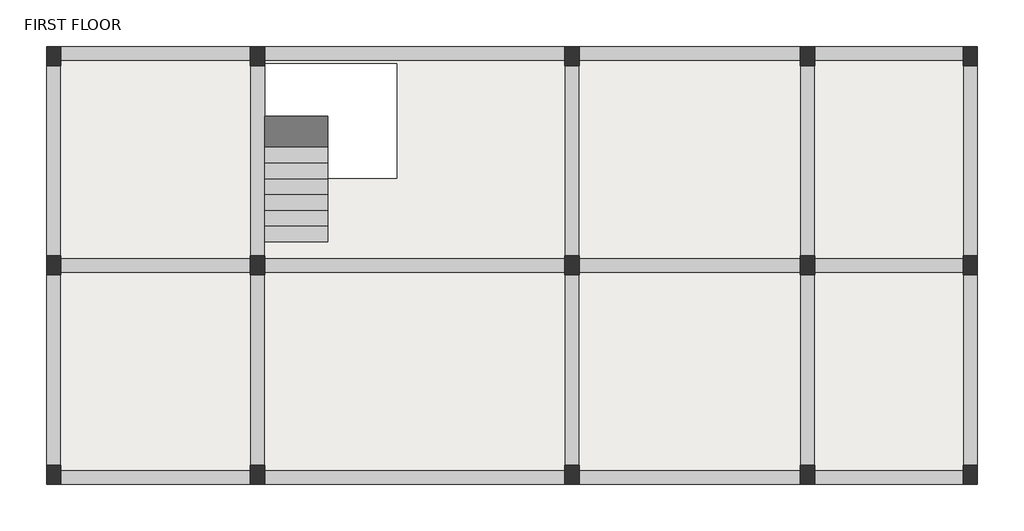
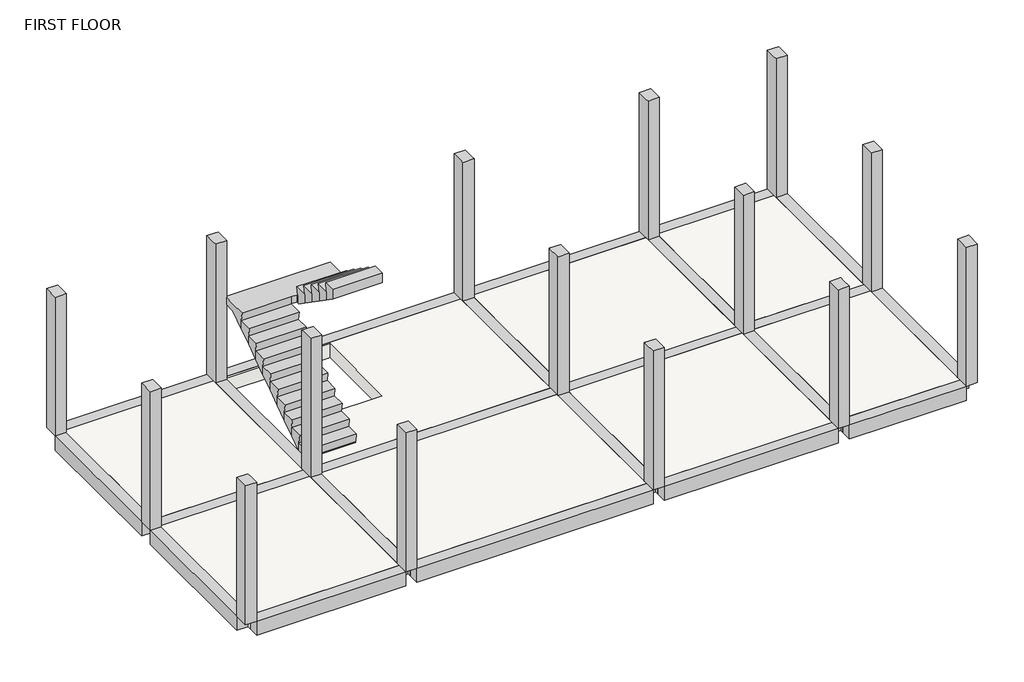
# One storey: 22 beams, 15 columns, 2 slabs, 1 stair flight.
"""IFC4 building model written with IfcOpenShell, lengths in millimetres."""

from ifc_helpers import new_model, si_unit, frame, origin, place, context, project, spatial, polyline, outline, extrude, faceted_brep, element, save

model = new_model("IFC4")

# Units and contexts
model_context = context("Model", 3, world=origin())
ifc_project = project(units=[si_unit("LENGTHUNIT", "METRE", prefix="MILLI")], contexts=[model_context])

# Site, building, storey
site = spatial("IfcSite", under=ifc_project)
building = spatial("IfcBuilding", under=site)
storey = spatial("IfcBuildingStorey", under=building, Name="FIRST FLOOR", Elevation=3000.0)

# Beams
placement = place(None, origin())
element("IfcBeam", 1, ObjectType="M_Concrete-Rectangular Beam : 100MM X 200MM", at=placement, inside=storey, context=model_context, shape_type="SweptSolid", body=[
    extrude(outline(polyline([(-5114.1068817, 5712.0180792), (-5342.7068817, 5712.0180792), (-5342.7068817, 8772.8765586), (-5114.1068817, 8772.8765586), (-5114.1068817, 5712.0180792)])), frame((0.0, 0.0, 2695.2), z_axis=(0.0, 0.0, 1.0), x_axis=(1.0, 0.0, 0.0)), (0.0, 0.0, 1.0), 304.8),
])
element("IfcBeam", 2, ObjectType="M_Concrete-Rectangular Beam : 100MM X 200MM", at=placement, inside=storey, context=model_context, shape_type="Brep", body=[
    faceted_brep([(-2066.1068817, 2041.8765586, 3000.0), (-2066.1068817, 2270.4765586, 3000.0), (-5114.1068817, 2270.4765586, 3000.0), (-5114.1068817, 2041.8765586, 3000.0), (-2066.1068817, 2041.8765586, 2695.2), (-5114.1068817, 2041.8765586, 2695.2), (-2066.1068817, 2270.4765586, 2695.2), (-5114.1068817, 2270.4765586, 2695.2), (-2066.1068817, 2270.4765586, 2700.0), (-5114.1068817, 2270.4765586, 2700.0)], [[[0, 1, 2, 3]], [[4, 0, 3, 5]], [[6, 4, 5, 7]], [[1, 8, 6, 7, 9, 2]], [[1, 0, 4, 6, 8]], [[3, 2, 9, 7, 5]]]),
])
element("IfcBeam", 3, ObjectType="M_Concrete-Rectangular Beam : 100MM X 200MM", at=placement, inside=storey, context=model_context, shape_type="SweptSolid", body=[
    extrude(outline(polyline([(-5114.1068817, 2346.6765586), (-5342.7068817, 2346.6765586), (-5342.7068817, 5407.2180792), (-5114.1068817, 5407.2180792), (-5114.1068817, 2346.6765586)])), frame((0.0, 0.0, 2695.2), z_axis=(0.0, 0.0, 1.0), x_axis=(1.0, 0.0, 0.0)), (0.0, 0.0, 1.0), 304.8),
])
element("IfcBeam", 4, ObjectType="M_Concrete-Rectangular Beam : 100MM X 200MM", at=placement, inside=storey, context=model_context, shape_type="Brep", body=[
    faceted_brep([(2988.1931183, 2041.8765586, 3000.0), (2988.1931183, 2270.4765586, 3000.0), (-1837.5068817, 2270.4765586, 3000.0), (-1837.5068817, 2041.8765586, 3000.0), (2988.1931183, 2041.8765586, 2695.2), (-1837.5068817, 2041.8765586, 2695.2), (2988.1931183, 2270.4765586, 2695.2), (-1837.5068817, 2270.4765586, 2695.2), (-1837.5068817, 2270.4765586, 2700.0)], [[[0, 1, 2, 3]], [[4, 0, 3, 5]], [[6, 4, 5, 7]], [[1, 6, 7, 8, 2]], [[1, 0, 4, 6]], [[3, 2, 8, 7, 5]]]),
])
element("IfcBeam", 5, ObjectType="M_Concrete-Rectangular Beam : 100MM X 200MM", at=placement, inside=storey, context=model_context, shape_type="Brep", body=[
    faceted_brep([(6773.0931183, 2041.8765586, 3000.0), (6773.0931183, 2270.4765586, 3000.0), (3217.0931183, 2270.4765586, 3000.0), (3217.0931183, 2041.8765586, 3000.0), (6773.0931183, 2041.8765586, 2695.2), (3217.0931183, 2041.8765586, 2695.2), (6773.0931183, 2270.4765586, 2695.2), (3217.0931183, 2270.4765586, 2695.2), (6773.0931183, 2270.4765586, 2700.0), (3217.0931183, 2270.4765586, 2700.0)], [[[0, 1, 2, 3]], [[4, 0, 3, 5]], [[6, 4, 5, 7]], [[1, 8, 6, 7, 9, 2]], [[1, 0, 4, 6, 8]], [[3, 2, 9, 7, 5]]]),
])
element("IfcBeam", 6, ObjectType="M_Concrete-Rectangular Beam : 100MM X 200MM", at=placement, inside=storey, context=model_context, shape_type="Brep", body=[
    faceted_brep([(9387.3931183, 2041.8765586, 3000.0), (9387.3931183, 2270.4765586, 3000.0), (7001.6931183, 2270.4765586, 3000.0), (7001.6931183, 2041.8765586, 3000.0), (9387.3931183, 2041.8765586, 2695.2), (7001.6931183, 2041.8765586, 2695.2), (9387.3931183, 2270.4765586, 2695.2), (7001.6931183, 2270.4765586, 2695.2), (7001.6931183, 2270.4765586, 2700.0)], [[[0, 1, 2, 3]], [[4, 0, 3, 5]], [[6, 4, 5, 7]], [[1, 6, 7, 8, 2]], [[1, 0, 4, 6]], [[3, 2, 8, 7, 5]]]),
])
element("IfcBeam", 7, ObjectType="M_Concrete-Rectangular Beam : 100MM X 200MM", at=placement, inside=storey, context=model_context, shape_type="Brep", body=[
    faceted_brep([(-2066.1068817, 8849.0765586, 3000.0), (-2066.1068817, 9077.6765586, 3000.0), (-5114.1068817, 9077.6765586, 3000.0), (-5114.1068817, 8849.0765586, 3000.0), (-2066.1068817, 8849.0765586, 2695.2), (-2066.1068817, 8849.0765586, 2700.0), (-5114.1068817, 8849.0765586, 2700.0), (-5114.1068817, 8849.0765586, 2695.2), (-2066.1068817, 9077.6765586, 2695.2), (-5114.1068817, 9077.6765586, 2695.2)], [[[0, 1, 2, 3]], [[4, 5, 0, 3, 6, 7]], [[8, 4, 7, 9]], [[1, 8, 9, 2]], [[1, 0, 5, 4, 8]], [[3, 2, 9, 7, 6]]]),
])
element("IfcBeam", 8, ObjectType="M_Concrete-Rectangular Beam : 100MM X 200MM", at=placement, inside=storey, context=model_context, shape_type="Brep", body=[
    faceted_brep([(2988.4931183, 8849.0765586, 3000.0), (2988.4931183, 9077.6765586, 3000.0), (-1837.5068817, 9077.6765586, 3000.0), (-1837.5068817, 8849.0765586, 3000.0), (2988.4931183, 8849.0765586, 2695.2), (2988.4931183, 8849.0765586, 2700.0), (-1837.5068817, 8849.0765586, 2700.0), (-1837.5068817, 8849.0765586, 2695.2), (2988.4931183, 9077.6765586, 2695.2), (-1837.5068817, 9077.6765586, 2695.2)], [[[0, 1, 2, 3]], [[4, 5, 0, 3, 6, 7]], [[8, 4, 7, 9]], [[1, 8, 9, 2]], [[1, 0, 5, 4, 8]], [[3, 2, 9, 7, 6]]]),
])
element("IfcBeam", 9, ObjectType="M_Concrete-Rectangular Beam : 100MM X 200MM", at=placement, inside=storey, context=model_context, shape_type="Brep", body=[
    faceted_brep([(6773.0931183, 8849.0765586, 3000.0), (6773.0931183, 9077.6765586, 3000.0), (3217.0931183, 9077.6765586, 3000.0), (3217.0931183, 8849.0765586, 3000.0), (6773.0931183, 8849.0765586, 2695.2), (6773.0931183, 8849.0765586, 2700.0), (3217.0931183, 8849.0765586, 2700.0), (3217.0931183, 8849.0765586, 2695.2), (6773.0931183, 9077.6765586, 2695.2), (3217.0931183, 9077.6765586, 2695.2)], [[[0, 1, 2, 3]], [[4, 5, 0, 3, 6, 7]], [[8, 4, 7, 9]], [[1, 8, 9, 2]], [[1, 0, 5, 4, 8]], [[3, 2, 9, 7, 6]]]),
])
element("IfcBeam", 10, ObjectType="M_Concrete-Rectangular Beam : 100MM X 200MM", at=placement, inside=storey, context=model_context, shape_type="Brep", body=[
    faceted_brep([(9387.3931183, 8849.0765586, 3000.0), (9387.3931183, 9077.6765586, 3000.0), (7001.6931183, 9077.6765586, 3000.0), (7001.6931183, 8849.0765586, 3000.0), (9387.3931183, 8849.0765586, 2695.2), (7001.6931183, 8849.0765586, 2700.0), (7001.6931183, 8849.0765586, 2695.2), (9387.3931183, 9077.6765586, 2695.2), (7001.6931183, 9077.6765586, 2695.2)], [[[0, 1, 2, 3]], [[4, 0, 3, 5, 6]], [[7, 4, 6, 8]], [[1, 7, 8, 2]], [[1, 0, 4, 7]], [[3, 2, 8, 6, 5]]]),
])
element("IfcBeam", 11, ObjectType="M_Concrete-Rectangular Beam : 100MM X 200MM", at=placement, inside=storey, context=model_context, shape_type="SweptSolid", body=[
    extrude(outline(polyline([(9617.8931183, 2354.2765586), (9389.2931183, 2354.2765586), (9389.2931183, 5407.2180792), (9617.8931183, 5407.2180792), (9617.8931183, 2354.2765586)])), frame((0.0, 0.0, 2695.2), z_axis=(0.0, 0.0, 1.0), x_axis=(1.0, 0.0, 0.0)), (0.0, 0.0, 1.0), 304.8),
])
element("IfcBeam", 12, ObjectType="M_Concrete-Rectangular Beam : 100MM X 200MM", at=placement, inside=storey, context=model_context, shape_type="SweptSolid", body=[
    extrude(outline(polyline([(9389.2931183, 8772.8765586), (9617.8931183, 8772.8765586), (9617.8931183, 5712.0180792), (9389.2931183, 5712.0180792), (9389.2931183, 8772.8765586)])), frame((0.0, 0.0, 2695.2), z_axis=(0.0, 0.0, 1.0), x_axis=(1.0, 0.0, 0.0)), (0.0, 0.0, 1.0), 304.8),
])
element("IfcBeam", 13, ObjectType="M_Concrete-Rectangular Beam : 100MM X 200MM", at=placement, inside=storey, context=model_context, shape_type="Brep", body=[
    faceted_brep([(7001.6931183, 5445.3180792, 3000.0), (9389.2931183, 5445.3180792, 3000.0), (9389.2931183, 5673.9180792, 3000.0), (7001.6931183, 5673.9180792, 3000.0), (9389.2931183, 5673.9180792, 2700.0), (9389.2931183, 5673.9180792, 2695.2), (7001.6931183, 5673.9180792, 2695.2), (7001.6931183, 5673.9180792, 2700.0), (9389.2931183, 5445.3180792, 2695.2), (7001.6931183, 5445.3180792, 2695.2), (7001.6931183, 5445.3180792, 2700.0), (9389.2931183, 5445.3180792, 2700.0)], [[[0, 1, 2, 3]], [[3, 2, 4, 5, 6, 7]], [[5, 8, 9, 6]], [[1, 0, 10, 9, 8, 11]], [[5, 4, 2, 1, 11, 8]], [[0, 3, 7, 6, 9, 10]]]),
])
element("IfcBeam", 14, ObjectType="M_Concrete-Rectangular Beam : 100MM X 200MM", at=placement, inside=storey, context=model_context, shape_type="Brep", body=[
    faceted_brep([(3217.0931183, 5445.3180792, 3000.0), (6773.0931183, 5445.3180792, 3000.0), (6773.0931183, 5673.9180792, 3000.0), (3217.0931183, 5673.9180792, 3000.0), (6773.0931183, 5673.9180792, 2700.0), (6773.0931183, 5673.9180792, 2695.2), (3217.0931183, 5673.9180792, 2695.2), (3217.0931183, 5673.9180792, 2700.0), (6773.0931183, 5445.3180792, 2695.2), (3217.0931183, 5445.3180792, 2695.2), (3217.0931183, 5445.3180792, 2700.0), (6773.0931183, 5445.3180792, 2700.0)], [[[0, 1, 2, 3]], [[3, 2, 4, 5, 6, 7]], [[5, 8, 9, 6]], [[1, 0, 10, 9, 8, 11]], [[2, 1, 11, 8, 5, 4]], [[0, 3, 7, 6, 9, 10]]]),
])
element("IfcBeam", 15, ObjectType="M_Concrete-Rectangular Beam : 100MM X 200MM", at=placement, inside=storey, context=model_context, shape_type="Brep", body=[
    faceted_brep([(-1837.5068817, 5445.3180792, 3000.0), (2988.4931183, 5445.3180792, 3000.0), (2988.4931183, 5673.9180792, 3000.0), (-1837.5068817, 5673.9180792, 3000.0), (2988.4931183, 5673.9180792, 2700.0), (2988.4931183, 5673.9180792, 2695.2), (-1837.5068817, 5673.9180792, 2695.2), (-1837.5068817, 5673.9180792, 2700.0), (2988.4931183, 5445.3180792, 2695.2), (-1837.5068817, 5445.3180792, 2695.2), (-1837.5068817, 5445.3180792, 2700.0), (2988.4931183, 5445.3180792, 2700.0)], [[[0, 1, 2, 3]], [[3, 2, 4, 5, 6, 7]], [[5, 8, 9, 6]], [[1, 0, 10, 9, 8, 11]], [[2, 1, 11, 8, 5, 4]], [[0, 3, 7, 6, 9, 10]]]),
])
element("IfcBeam", 16, ObjectType="M_Concrete-Rectangular Beam : 100MM X 200MM", at=placement, inside=storey, context=model_context, shape_type="Brep", body=[
    faceted_brep([(-2066.1068817, 5673.9180792, 3000.0), (-5114.1068817, 5673.9180792, 3000.0), (-5114.1068817, 5445.3180792, 3000.0), (-2066.1068817, 5445.3180792, 3000.0), (-2066.1068817, 5673.9180792, 2700.0), (-2066.1068817, 5673.9180792, 2695.2), (-5114.1068817, 5673.9180792, 2695.2), (-5114.1068817, 5673.9180792, 2700.0), (-2066.1068817, 5445.3180792, 2695.2), (-5114.1068817, 5445.3180792, 2695.2), (-2066.1068817, 5445.3180792, 2700.0), (-5114.1068817, 5445.3180792, 2700.0)], [[[0, 1, 2, 3]], [[1, 0, 4, 5, 6, 7]], [[5, 8, 9, 6]], [[8, 10, 3, 2, 11, 9]], [[0, 3, 10, 8, 5, 4]], [[2, 1, 7, 6, 9, 11]]]),
])
element("IfcBeam", 17, ObjectType="M_Concrete-Rectangular Beam : 100MM X 200MM", at=placement, inside=storey, context=model_context, shape_type="SweptSolid", body=[
    extrude(outline(polyline([(6773.0931183, 5407.2180792), (7001.6931183, 5407.2180792), (7001.6931183, 2346.6765586), (6773.0931183, 2346.6765586), (6773.0931183, 5407.2180792)])), frame((0.0, 0.0, 2695.2), z_axis=(0.0, 0.0, 1.0), x_axis=(1.0, 0.0, 0.0)), (0.0, 0.0, 1.0), 304.8),
])
element("IfcBeam", 18, ObjectType="M_Concrete-Rectangular Beam : 100MM X 200MM", at=placement, inside=storey, context=model_context, shape_type="SweptSolid", body=[
    extrude(outline(polyline([(6773.0931183, 8772.8765586), (7001.6931183, 8772.8765586), (7001.6931183, 5712.0180792), (6773.0931183, 5712.0180792), (6773.0931183, 8772.8765586)])), frame((0.0, 0.0, 2695.2), z_axis=(0.0, 0.0, 1.0), x_axis=(1.0, 0.0, 0.0)), (0.0, 0.0, 1.0), 304.8),
])
element("IfcBeam", 19, ObjectType="M_Concrete-Rectangular Beam : 100MM X 200MM", at=placement, inside=storey, context=model_context, shape_type="SweptSolid", body=[
    extrude(outline(polyline([(2988.4931183, 5407.2180792), (3217.0931183, 5407.2180792), (3217.0931183, 2346.6765586), (2988.4931183, 2346.6765586), (2988.4931183, 5407.2180792)])), frame((0.0, 0.0, 2695.2), z_axis=(0.0, 0.0, 1.0), x_axis=(1.0, 0.0, 0.0)), (0.0, 0.0, 1.0), 304.8),
])
element("IfcBeam", 20, ObjectType="M_Concrete-Rectangular Beam : 100MM X 200MM", at=placement, inside=storey, context=model_context, shape_type="Brep", body=[
    faceted_brep([(2988.4931183, 5719.6180792, 3000.0), (3217.0931183, 5719.6180792, 3000.0), (3217.0931183, 8772.8765586, 3000.0), (2988.4931183, 8772.8765586, 3000.0), (3217.0931183, 5719.6180792, 2700.0), (3217.0931183, 5719.6180792, 2695.2), (3217.0931183, 8772.8765586, 2695.2), (2988.4931183, 5719.6180792, 2695.2), (2988.4931183, 8772.8765586, 2695.2), (2988.4931183, 5719.6180792, 2700.0)], [[[0, 1, 2, 3]], [[1, 4, 5, 6, 2]], [[5, 7, 8, 6]], [[7, 9, 0, 3, 8]], [[7, 5, 4, 1, 0, 9]], [[3, 2, 6, 8]]]),
])
element("IfcBeam", 21, ObjectType="M_Concrete-Rectangular Beam : 100MM X 200MM", at=placement, inside=storey, context=model_context, shape_type="SweptSolid", body=[
    extrude(outline(polyline([(-2066.1068817, 5407.2180792), (-1837.5068817, 5407.2180792), (-1837.5068817, 2346.6765586), (-2066.1068817, 2346.6765586), (-2066.1068817, 5407.2180792)])), frame((0.0, 0.0, 2695.2), z_axis=(0.0, 0.0, 1.0), x_axis=(1.0, 0.0, 0.0)), (0.0, 0.0, 1.0), 304.8),
])
element("IfcBeam", 22, ObjectType="M_Concrete-Rectangular Beam : 100MM X 200MM", at=placement, inside=storey, context=model_context, shape_type="Brep", body=[
    faceted_brep([(-1837.5068817, 8772.8765586, 3000.0), (-2066.1068817, 8772.8765586, 3000.0), (-2066.1068817, 5712.0180792, 3000.0), (-1837.5068817, 5712.0180792, 3000.0), (-1837.5068817, 5940.7765586, 3000.0), (-1837.5068817, 8772.8765586, 2695.2), (-1837.5068817, 5712.0180792, 2695.2), (-2066.1068817, 8772.8765586, 2695.2), (-2066.1068817, 5712.0180792, 2695.2)], [[[0, 1, 2, 3, 4]], [[5, 0, 4, 3, 6]], [[7, 5, 6, 8]], [[1, 7, 8, 2]], [[1, 0, 5, 7]], [[3, 2, 8, 6]]]),
])

# Columns
element("IfcColumn", 23, ObjectType="M_Concrete-Rectangular-Column : 9\" X 1' COLUMNS", at=placement, inside=storey, context=model_context, shape_type="Brep", body=[
    faceted_brep([(9617.8931183, 9077.6765586, 3000.0), (9617.8931183, 8772.8765586, 3000.0), (9389.2931183, 8772.8765586, 3000.0), (9389.2931183, 9077.6765586, 3000.0), (9617.8931183, 9077.6765586, 6000.0), (9617.8931183, 8772.8765586, 6000.0), (9389.2931183, 8772.8765586, 6000.0), (9389.2931183, 8849.0765586, 6000.0), (9389.2931183, 9077.6765586, 6000.0)], [[[0, 1, 2, 3]], [[4, 5, 1, 0]], [[5, 6, 2, 1]], [[6, 7, 8, 3, 2]], [[8, 4, 0, 3]], [[4, 8, 7, 6, 5]]]),
])
element("IfcColumn", 24, ObjectType="M_Concrete-Rectangular-Column : 9\" X 1' COLUMNS", at=placement, inside=storey, context=model_context, shape_type="Brep", body=[
    faceted_brep([(9617.8931183, 5712.0180792, 3000.0), (9617.8931183, 5407.2180792, 3000.0), (9389.2931183, 5407.2180792, 3000.0), (9389.2931183, 5712.0180792, 3000.0), (9617.8931183, 5712.0180792, 6000.0), (9617.8931183, 5407.2180792, 6000.0), (9389.2931183, 5407.2180792, 6000.0), (9389.2931183, 5445.3180792, 6000.0), (9389.2931183, 5673.9180792, 6000.0), (9389.2931183, 5712.0180792, 6000.0)], [[[0, 1, 2, 3]], [[4, 5, 1, 0]], [[5, 6, 2, 1]], [[6, 7, 8, 9, 3, 2]], [[9, 4, 0, 3]], [[4, 9, 8, 7, 6, 5]]]),
])
element("IfcColumn", 25, ObjectType="M_Concrete-Rectangular-Column : 9\" X 1' COLUMNS", at=placement, inside=storey, context=model_context, shape_type="Brep", body=[
    faceted_brep([(9617.8931183, 2346.6765586, 3000.0), (9617.8931183, 2041.8765586, 3000.0), (9389.2931183, 2041.8765586, 3000.0), (9389.2931183, 2346.6765586, 3000.0), (9617.8931183, 2346.6765586, 6000.0), (9617.8931183, 2041.8765586, 6000.0), (9389.2931183, 2041.8765586, 6000.0), (9389.2931183, 2270.4765586, 6000.0), (9389.2931183, 2346.6765586, 6000.0)], [[[0, 1, 2, 3]], [[4, 5, 1, 0]], [[5, 6, 2, 1]], [[6, 7, 8, 3, 2]], [[8, 4, 0, 3]], [[4, 8, 7, 6, 5]]]),
])
element("IfcColumn", 26, ObjectType="M_Concrete-Rectangular-Column : 9\" X 1' COLUMNS", at=placement, inside=storey, context=model_context, shape_type="Brep", body=[
    faceted_brep([(7001.6931183, 9077.6765586, 3000.0), (7001.6931183, 8772.8765586, 3000.0), (6773.0931183, 8772.8765586, 3000.0), (6773.0931183, 9077.6765586, 3000.0), (7001.6931183, 9077.6765586, 6000.0), (7001.6931183, 8849.0765586, 6000.0), (7001.6931183, 8772.8765586, 6000.0), (7001.6931183, 8772.8765586, 5700.0), (6773.0931183, 8772.8765586, 6000.0), (6773.0931183, 8772.8765586, 5700.0), (6773.0931183, 8849.0765586, 6000.0), (6773.0931183, 9077.6765586, 6000.0)], [[[0, 1, 2, 3]], [[1, 0, 4, 5, 6, 7]], [[2, 1, 7, 6, 8, 9]], [[3, 2, 9, 8, 10, 11]], [[0, 3, 11, 4]], [[8, 6, 5, 4, 11, 10]]]),
])
element("IfcColumn", 27, ObjectType="M_Concrete-Rectangular-Column : 9\" X 1' COLUMNS", at=placement, inside=storey, context=model_context, shape_type="Brep", body=[
    faceted_brep([(7001.6931183, 5712.0180792, 3000.0), (7001.6931183, 5407.2180792, 3000.0), (6773.0931183, 5407.2180792, 3000.0), (6773.0931183, 5712.0180792, 3000.0), (7001.6931183, 5712.0180792, 5700.0), (7001.6931183, 5712.0180792, 6000.0), (7001.6931183, 5673.9180792, 6000.0), (7001.6931183, 5445.3180792, 6000.0), (7001.6931183, 5407.2180792, 6000.0), (7001.6931183, 5407.2180792, 5700.0), (6773.0931183, 5407.2180792, 6000.0), (6773.0931183, 5407.2180792, 5700.0), (6773.0931183, 5445.3180792, 6000.0), (6773.0931183, 5673.9180792, 6000.0), (6773.0931183, 5712.0180792, 6000.0), (6773.0931183, 5712.0180792, 5700.0)], [[[0, 1, 2, 3]], [[1, 0, 4, 5, 6, 7, 8, 9]], [[2, 1, 9, 8, 10, 11]], [[3, 2, 11, 10, 12, 13, 14, 15]], [[0, 3, 15, 14, 5, 4]], [[10, 8, 7, 6, 5, 14, 13, 12]]]),
])
element("IfcColumn", 28, ObjectType="M_Concrete-Rectangular-Column : 9\" X 1' COLUMNS", at=placement, inside=storey, context=model_context, shape_type="Brep", body=[
    faceted_brep([(7001.6931183, 2346.6765586, 3000.0), (7001.6931183, 2041.8765586, 3000.0), (6773.0931183, 2041.8765586, 3000.0), (6773.0931183, 2346.6765586, 3000.0), (7001.6931183, 2346.6765586, 5700.0), (7001.6931183, 2346.6765586, 6000.0), (7001.6931183, 2270.4765586, 6000.0), (7001.6931183, 2041.8765586, 6000.0), (6773.0931183, 2041.8765586, 6000.0), (6773.0931183, 2270.4765586, 6000.0), (6773.0931183, 2346.6765586, 6000.0), (6773.0931183, 2346.6765586, 5700.0)], [[[0, 1, 2, 3]], [[1, 0, 4, 5, 6, 7]], [[2, 1, 7, 8]], [[3, 2, 8, 9, 10, 11]], [[0, 3, 11, 10, 5, 4]], [[8, 7, 6, 5, 10, 9]]]),
])
element("IfcColumn", 29, ObjectType="M_Concrete-Rectangular-Column : 9\" X 1' COLUMNS", at=placement, inside=storey, context=model_context, shape_type="Brep", body=[
    faceted_brep([(3217.0931183, 9077.6765586, 3000.0), (3217.0931183, 8772.8765586, 3000.0), (2988.4931183, 8772.8765586, 3000.0), (2988.4931183, 9077.6765586, 3000.0), (3217.0931183, 9077.6765586, 6000.0), (3217.0931183, 8849.0765586, 6000.0), (3217.0931183, 8772.8765586, 6000.0), (3217.0931183, 8772.8765586, 5700.0), (2988.4931183, 8772.8765586, 6000.0), (2988.4931183, 8772.8765586, 5700.0), (2988.4931183, 8849.0765586, 6000.0), (2988.4931183, 9077.6765586, 6000.0)], [[[0, 1, 2, 3]], [[1, 0, 4, 5, 6, 7]], [[2, 1, 7, 6, 8, 9]], [[3, 2, 9, 8, 10, 11]], [[0, 3, 11, 4]], [[8, 6, 5, 4, 11, 10]]]),
])
element("IfcColumn", 30, ObjectType="M_Concrete-Rectangular-Column : 9\" X 1' COLUMNS", at=placement, inside=storey, context=model_context, shape_type="Brep", body=[
    faceted_brep([(3217.0931183, 5712.0180792, 3000.0), (3217.0931183, 5407.2180792, 3000.0), (2988.4931183, 5407.2180792, 3000.0), (2988.4931183, 5712.0180792, 3000.0), (3217.0931183, 5712.0180792, 5700.0), (3217.0931183, 5712.0180792, 6000.0), (3217.0931183, 5673.9180792, 6000.0), (3217.0931183, 5445.3180792, 6000.0), (3217.0931183, 5407.2180792, 6000.0), (3217.0931183, 5407.2180792, 5700.0), (2988.4931183, 5407.2180792, 6000.0), (2988.4931183, 5407.2180792, 5700.0), (2988.4931183, 5445.3180792, 6000.0), (2988.4931183, 5673.9180792, 6000.0), (2988.4931183, 5712.0180792, 6000.0), (2988.4931183, 5712.0180792, 5700.0)], [[[0, 1, 2, 3]], [[1, 0, 4, 5, 6, 7, 8, 9]], [[2, 1, 9, 8, 10, 11]], [[3, 2, 11, 10, 12, 13, 14, 15]], [[0, 3, 15, 14, 5, 4]], [[10, 8, 7, 6, 5, 14, 13, 12]]]),
])
element("IfcColumn", 31, ObjectType="M_Concrete-Rectangular-Column : 9\" X 1' COLUMNS", at=placement, inside=storey, context=model_context, shape_type="Brep", body=[
    faceted_brep([(3217.0931183, 2346.6765586, 3000.0), (3217.0931183, 2041.8765586, 3000.0), (2988.4931183, 2041.8765586, 3000.0), (2988.4931183, 2346.6765586, 3000.0), (3217.0931183, 2346.6765586, 5700.0), (3217.0931183, 2346.6765586, 6000.0), (3217.0931183, 2270.4765586, 6000.0), (3217.0931183, 2041.8765586, 6000.0), (2988.4931183, 2041.8765586, 6000.0), (2988.4931183, 2270.4765586, 6000.0), (2988.4931183, 2346.6765586, 6000.0), (2988.4931183, 2346.6765586, 5700.0)], [[[0, 1, 2, 3]], [[1, 0, 4, 5, 6, 7]], [[2, 1, 7, 8]], [[3, 2, 8, 9, 10, 11]], [[0, 3, 11, 10, 5, 4]], [[8, 7, 6, 5, 10, 9]]]),
])
element("IfcColumn", 32, ObjectType="M_Concrete-Rectangular-Column : 9\" X 1' COLUMNS", at=placement, inside=storey, context=model_context, shape_type="Brep", body=[
    faceted_brep([(-1837.5068817, 9077.6765586, 3000.0), (-1837.5068817, 8772.8765586, 3000.0), (-2066.1068817, 8772.8765586, 3000.0), (-2066.1068817, 9077.6765586, 3000.0), (-1837.5068817, 9077.6765586, 6000.0), (-1837.5068817, 8849.0765586, 6000.0), (-1837.5068817, 8810.9765586, 6000.0), (-1837.5068817, 8772.8765586, 6000.0), (-2066.1068817, 8772.8765586, 6000.0), (-2066.1068817, 8772.8765586, 5700.0), (-2066.1068817, 8849.0765586, 6000.0), (-2066.1068817, 9077.6765586, 6000.0)], [[[0, 1, 2, 3]], [[1, 0, 4, 5, 6, 7]], [[2, 1, 7, 8, 9]], [[3, 2, 9, 8, 10, 11]], [[0, 3, 11, 4]], [[8, 7, 6, 5, 4, 11, 10]]]),
])
element("IfcColumn", 33, ObjectType="M_Concrete-Rectangular-Column : 9\" X 1' COLUMNS", at=placement, inside=storey, context=model_context, shape_type="Brep", body=[
    faceted_brep([(-1837.5068817, 5712.0180792, 3000.0), (-1837.5068817, 5407.2180792, 3000.0), (-2066.1068817, 5407.2180792, 3000.0), (-2066.1068817, 5712.0180792, 3000.0), (-1837.5068817, 5712.0180792, 5700.0), (-1837.5068817, 5712.0180792, 6000.0), (-1837.5068817, 5673.9180792, 6000.0), (-1837.5068817, 5445.3180792, 6000.0), (-1837.5068817, 5407.2180792, 6000.0), (-1837.5068817, 5407.2180792, 5700.0), (-2066.1068817, 5407.2180792, 6000.0), (-2066.1068817, 5445.3180792, 6000.0), (-2066.1068817, 5673.9180792, 6000.0), (-2066.1068817, 5712.0180792, 6000.0), (-2066.1068817, 5712.0180792, 5700.0)], [[[0, 1, 2, 3]], [[1, 0, 4, 5, 6, 7, 8, 9]], [[2, 1, 9, 8, 10]], [[3, 2, 10, 11, 12, 13, 14]], [[0, 3, 14, 13, 5, 4]], [[10, 8, 7, 6, 5, 13, 12, 11]]]),
])
element("IfcColumn", 34, ObjectType="M_Concrete-Rectangular-Column : 9\" X 1' COLUMNS", at=placement, inside=storey, context=model_context, shape_type="Brep", body=[
    faceted_brep([(-1837.5068817, 2346.6765586, 3000.0), (-1837.5068817, 2041.8765586, 3000.0), (-2066.1068817, 2041.8765586, 3000.0), (-2066.1068817, 2346.6765586, 3000.0), (-1837.5068817, 2346.6765586, 5700.0), (-1837.5068817, 2346.6765586, 6000.0), (-1837.5068817, 2270.4765586, 6000.0), (-1837.5068817, 2041.8765586, 6000.0), (-2066.1068817, 2041.8765586, 6000.0), (-2066.1068817, 2270.4765586, 6000.0), (-2066.1068817, 2346.6765586, 6000.0)], [[[0, 1, 2, 3]], [[1, 0, 4, 5, 6, 7]], [[2, 1, 7, 8]], [[3, 2, 8, 9, 10]], [[0, 3, 10, 5, 4]], [[8, 7, 6, 5, 10, 9]]]),
])
element("IfcColumn", 35, ObjectType="M_Concrete-Rectangular-Column : 9\" X 1' COLUMNS", at=placement, inside=storey, context=model_context, shape_type="Brep", body=[
    faceted_brep([(-5114.1068817, 2346.6765586, 3000.0), (-5114.1068817, 2041.8765586, 3000.0), (-5342.7068817, 2041.8765586, 3000.0), (-5342.7068817, 2346.6765586, 3000.0), (-5114.1068817, 2346.6765586, 6000.0), (-5114.1068817, 2270.4765586, 6000.0), (-5114.1068817, 2041.8765586, 6000.0), (-5342.7068817, 2041.8765586, 6000.0), (-5342.7068817, 2346.6765586, 6000.0)], [[[0, 1, 2, 3]], [[4, 5, 6, 1, 0]], [[6, 7, 2, 1]], [[7, 8, 3, 2]], [[8, 4, 0, 3]], [[4, 8, 7, 6, 5]]]),
])
element("IfcColumn", 36, ObjectType="M_Concrete-Rectangular-Column : 9\" X 1' COLUMNS", at=placement, inside=storey, context=model_context, shape_type="Brep", body=[
    faceted_brep([(-5114.1068817, 5712.0180792, 3000.0), (-5114.1068817, 5407.2180792, 3000.0), (-5342.7068817, 5407.2180792, 3000.0), (-5342.7068817, 5712.0180792, 3000.0), (-5114.1068817, 5712.0180792, 6000.0), (-5114.1068817, 5673.9180792, 6000.0), (-5114.1068817, 5445.3180792, 6000.0), (-5114.1068817, 5407.2180792, 6000.0), (-5342.7068817, 5407.2180792, 6000.0), (-5342.7068817, 5712.0180792, 6000.0)], [[[0, 1, 2, 3]], [[4, 5, 6, 7, 1, 0]], [[7, 8, 2, 1]], [[8, 9, 3, 2]], [[9, 4, 0, 3]], [[4, 9, 8, 7, 6, 5]]]),
])
element("IfcColumn", 37, ObjectType="M_Concrete-Rectangular-Column : 9\" X 1' COLUMNS", at=placement, inside=storey, context=model_context, shape_type="Brep", body=[
    faceted_brep([(-5114.1068817, 9077.6765586, 3000.0), (-5114.1068817, 8772.8765586, 3000.0), (-5342.7068817, 8772.8765586, 3000.0), (-5342.7068817, 9077.6765586, 3000.0), (-5114.1068817, 9077.6765586, 6000.0), (-5114.1068817, 8849.0765586, 6000.0), (-5114.1068817, 8772.8765586, 6000.0), (-5342.7068817, 8772.8765586, 6000.0), (-5342.7068817, 9077.6765586, 6000.0)], [[[0, 1, 2, 3]], [[4, 5, 6, 1, 0]], [[6, 7, 2, 1]], [[7, 8, 3, 2]], [[8, 4, 0, 3]], [[4, 8, 7, 6, 5]]]),
])

# Slabs
element("IfcSlab", 38, ObjectType="Generic 300mm", at=placement, inside=storey, context=model_context, shape_type="Brep", body=[
    faceted_brep([(-2066.1068817, 2270.4765586, 2700.0), (-5114.1068817, 2270.4765586, 2700.0), (-5114.1068817, 5445.3180792, 2700.0), (-2066.1068817, 5445.3180792, 2700.0), (-2066.1068817, 2270.4765586, 3000.0), (-2066.1068817, 2346.6765586, 3000.0), (-2066.1068817, 5407.2180792, 3000.0), (-2066.1068817, 5445.3180792, 3000.0), (-5114.1068817, 5445.3180792, 3000.0), (-5114.1068817, 5407.2180792, 3000.0), (-5114.1068817, 2346.6765586, 3000.0), (-5114.1068817, 2270.4765586, 3000.0)], [[[0, 1, 2, 3]], [[4, 5, 6, 7, 8, 9, 10, 11]], [[1, 0, 4, 11]], [[2, 1, 11, 10, 9, 8]], [[3, 2, 8, 7]], [[0, 3, 7, 6, 5, 4]]]),
])
element("IfcSlab", 39, ObjectType="Generic 300mm", at=placement, inside=storey, context=model_context, shape_type="Brep", body=[
    faceted_brep([(2988.4931183, 2270.4765586, 2700.0), (-1837.5068817, 2270.4765586, 2700.0), (-1837.5068817, 5445.3180792, 2700.0), (2988.4931183, 5445.3180792, 2700.0), (-1837.5068817, 2270.4765586, 3000.0), (2988.1931183, 2270.4765586, 3000.0), (2988.4931183, 2270.4765586, 3000.0), (2988.4931183, 2346.6765586, 3000.0), (2988.4931183, 5407.2180792, 3000.0), (2988.4931183, 5445.3180792, 3000.0), (-1837.5068817, 5445.3180792, 3000.0), (-1837.5068817, 5407.2180792, 3000.0), (-1837.5068817, 2346.6765586, 3000.0)], [[[0, 1, 2, 3]], [[4, 5, 6, 7, 8, 9, 10, 11, 12]], [[1, 0, 6, 5, 4]], [[2, 1, 4, 12, 11, 10]], [[3, 2, 10, 9]], [[0, 3, 9, 8, 7, 6]]]),
    faceted_brep([(6773.0931183, 2270.4765586, 2700.0), (3217.0931183, 2270.4765586, 2700.0), (3217.0931183, 5445.3180792, 2700.0), (6773.0931183, 5445.3180792, 2700.0), (3217.0931183, 2270.4765586, 3000.0), (6773.0931183, 2270.4765586, 3000.0), (6773.0931183, 2346.6765586, 3000.0), (6773.0931183, 5407.2180792, 3000.0), (6773.0931183, 5445.3180792, 3000.0), (3217.0931183, 5445.3180792, 3000.0), (3217.0931183, 5407.2180792, 3000.0), (3217.0931183, 2346.6765586, 3000.0)], [[[0, 1, 2, 3]], [[4, 5, 6, 7, 8, 9, 10, 11]], [[1, 0, 5, 4]], [[2, 1, 4, 11, 10, 9]], [[3, 2, 9, 8]], [[0, 3, 8, 7, 6, 5]]]),
    faceted_brep([(9389.2931183, 2270.4765586, 2700.0), (7001.6931183, 2270.4765586, 2700.0), (7001.6931183, 5445.3180792, 2700.0), (9389.2931183, 5445.3180792, 2700.0), (7001.6931183, 2270.4765586, 3000.0), (9387.3931183, 2270.4765586, 3000.0), (9389.2931183, 2270.4765586, 3000.0), (9389.2931183, 2346.6765586, 3000.0), (9389.2931183, 2354.2765586, 3000.0), (9389.2931183, 5407.2180792, 3000.0), (9389.2931183, 5445.3180792, 3000.0), (7001.6931183, 5445.3180792, 3000.0), (7001.6931183, 5407.2180792, 3000.0), (7001.6931183, 2346.6765586, 3000.0)], [[[0, 1, 2, 3]], [[4, 5, 6, 7, 8, 9, 10, 11, 12, 13]], [[1, 0, 6, 5, 4]], [[2, 1, 4, 13, 12, 11]], [[3, 2, 11, 10]], [[0, 3, 10, 9, 8, 7, 6]]]),
    faceted_brep([(7001.6931183, 5673.9180792, 2700.0), (7001.6931183, 8849.0765586, 2700.0), (9389.2931183, 8849.0765586, 2700.0), (9389.2931183, 5673.9180792, 2700.0), (7001.6931183, 8849.0765586, 3000.0), (7001.6931183, 8772.8765586, 3000.0), (7001.6931183, 5712.0180792, 3000.0), (7001.6931183, 5673.9180792, 3000.0), (9389.2931183, 5673.9180792, 3000.0), (9389.2931183, 5712.0180792, 3000.0), (9389.2931183, 8772.8765586, 3000.0), (9389.2931183, 8849.0765586, 3000.0), (9387.3931183, 8849.0765586, 3000.0)], [[[0, 1, 2, 3]], [[4, 5, 6, 7, 8, 9, 10, 11, 12]], [[1, 0, 7, 6, 5, 4]], [[2, 1, 4, 12, 11]], [[3, 2, 11, 10, 9, 8]], [[0, 3, 8, 7]]]),
    faceted_brep([(3217.0931183, 5673.9180792, 2700.0), (3217.0931183, 8849.0765586, 2700.0), (6773.0931183, 8849.0765586, 2700.0), (6773.0931183, 5673.9180792, 2700.0), (3217.0931183, 8849.0765586, 3000.0), (3217.0931183, 8772.8765586, 3000.0), (3217.0931183, 5719.6180792, 3000.0), (3217.0931183, 5712.0180792, 3000.0), (3217.0931183, 5673.9180792, 3000.0), (6773.0931183, 5673.9180792, 3000.0), (6773.0931183, 5712.0180792, 3000.0), (6773.0931183, 8772.8765586, 3000.0), (6773.0931183, 8849.0765586, 3000.0)], [[[0, 1, 2, 3]], [[4, 5, 6, 7, 8, 9, 10, 11, 12]], [[1, 0, 8, 7, 6, 5, 4]], [[2, 1, 4, 12]], [[3, 2, 12, 11, 10, 9]], [[0, 3, 9, 8]]]),
    faceted_brep([(-1837.5068817, 8849.0765586, 2700.0), (2988.4931183, 8849.0765586, 2700.0), (2988.4931183, 5673.9180792, 2700.0), (-1837.5068817, 5673.9180792, 2700.0), (-1837.5068817, 5940.7765586, 2700.0), (-821.5068817, 5940.7765586, 2700.0), (-821.5068817, 6956.7765586, 2700.0), (296.0931183, 6956.7765586, 2700.0), (296.0931183, 8810.9765586, 2700.0), (-1837.5068817, 8810.9765586, 2700.0), (2988.4931183, 8849.0765586, 3000.0), (-1837.5068817, 8849.0765586, 3000.0), (-1837.5068817, 8810.9765586, 3000.0), (296.0931183, 8810.9765586, 3000.0), (296.0931183, 6956.7765586, 3000.0), (-821.5068817, 6956.7765586, 3000.0), (-821.5068817, 5940.7765586, 3000.0), (-1837.5068817, 5940.7765586, 3000.0), (-1837.5068817, 5712.0180792, 3000.0), (-1837.5068817, 5673.9180792, 3000.0), (2988.4931183, 5673.9180792, 3000.0), (2988.4931183, 5712.0180792, 3000.0), (2988.4931183, 5719.6180792, 3000.0), (2988.4931183, 8772.8765586, 3000.0)], [[[0, 1, 2, 3, 4, 5, 6, 7, 8, 9]], [[10, 11, 12, 13, 14, 15, 16, 17, 18, 19, 20, 21, 22, 23]], [[3, 19, 18, 17, 4]], [[11, 0, 9, 12]], [[1, 0, 11, 10]], [[2, 1, 10, 23, 22, 21, 20]], [[3, 2, 20, 19]], [[5, 16, 15, 6]], [[6, 15, 14, 7]], [[7, 14, 13, 8]], [[8, 13, 12, 9]], [[16, 5, 4, 17]]]),
    faceted_brep([(-5114.1068817, 5673.9180792, 2700.0), (-5114.1068817, 8849.0765586, 2700.0), (-2066.1068817, 8849.0765586, 2700.0), (-2066.1068817, 5673.9180792, 2700.0), (-5114.1068817, 8849.0765586, 3000.0), (-5114.1068817, 8772.8765586, 3000.0), (-5114.1068817, 5712.0180792, 3000.0), (-5114.1068817, 5673.9180792, 3000.0), (-2066.1068817, 5673.9180792, 3000.0), (-2066.1068817, 5712.0180792, 3000.0), (-2066.1068817, 8772.8765586, 3000.0), (-2066.1068817, 8849.0765586, 3000.0)], [[[0, 1, 2, 3]], [[4, 5, 6, 7, 8, 9, 10, 11]], [[1, 0, 7, 6, 5, 4]], [[2, 1, 4, 11]], [[3, 2, 11, 10, 9, 8]], [[0, 3, 8, 7]]]),
])

# Stair flight
element("IfcStairFlight", 40, ObjectType="25 mm Nosing", at=placement, inside=storey, context=model_context, shape_type="Brep", body=[
    faceted_brep([(-1837.5068817, 5940.7765586, 3176.4705882), (-821.5068817, 5940.7765586, 3176.4705882), (-821.5068817, 6219.7765586, 3176.4705882), (-1837.5068817, 6219.7765586, 3176.4705882), (-1837.5068817, 6219.7765586, 3000.0), (-1837.5068817, 5965.7765586, 3000.0), (-821.5068817, 5965.7765586, 3000.0), (-821.5068817, 6219.7765586, 3000.0), (-1837.5068817, 6194.7765586, 3352.9411765), (-821.5068817, 6194.7765586, 3352.9411765), (-821.5068817, 6473.7765586, 3352.9411765), (-1837.5068817, 6473.7765586, 3352.9411765), (-1837.5068817, 6473.7765586, 3170.2919269), (-1837.5068817, 6228.6697118, 3000.0), (-821.5068817, 6228.6697118, 3000.0), (-821.5068817, 6473.7765586, 3170.2919269), (-1837.5068817, 6448.7765586, 3529.4117647), (-821.5068817, 6448.7765586, 3529.4117647), (-821.5068817, 6727.7765586, 3529.4117647), (-1837.5068817, 6727.7765586, 3529.4117647), (-1837.5068817, 6727.7765586, 3346.7625151), (-821.5068817, 6727.7765586, 3346.7625151), (-1837.5068817, 6702.7765586, 3705.8823529), (-821.5068817, 6702.7765586, 3705.8823529), (-821.5068817, 6981.7765586, 3705.8823529), (-1837.5068817, 6981.7765586, 3705.8823529), (-1837.5068817, 6981.7765586, 3523.2331034), (-821.5068817, 6981.7765586, 3523.2331034), (-1837.5068817, 6956.7765586, 3882.3529412), (-821.5068817, 6956.7765586, 3882.3529412), (-821.5068817, 7235.7765586, 3882.3529412), (-1837.5068817, 7235.7765586, 3882.3529412), (-1837.5068817, 7235.7765586, 3699.7036916), (-821.5068817, 7235.7765586, 3699.7036916), (-1837.5068817, 7210.7765586, 4058.8235294), (-821.5068817, 7210.7765586, 4058.8235294), (-821.5068817, 7489.7765586, 4058.8235294), (-1837.5068817, 7489.7765586, 4058.8235294), (-1837.5068817, 7489.7765586, 3876.1742799), (-821.5068817, 7489.7765586, 3876.1742799), (-1837.5068817, 7464.7765586, 4235.2941176), (-821.5068817, 7464.7765586, 4235.2941176), (-821.5068817, 7743.7765586, 4235.2941176), (-1837.5068817, 7743.7765586, 4235.2941176), (-1837.5068817, 7743.7765586, 4052.6448681), (-821.5068817, 7743.7765586, 4052.6448681), (-1837.5068817, 7718.7765586, 4411.7647059), (-821.5068817, 7718.7765586, 4411.7647059), (-821.5068817, 7997.7765586, 4411.7647059), (-1837.5068817, 7997.7765586, 4411.7647059), (-1837.5068817, 7997.7765586, 4229.1154563), (-821.5068817, 7997.7765586, 4229.1154563), (-1837.5068817, 7972.7765586, 4588.2352941), (-821.5068817, 7972.7765586, 4588.2352941), (-821.5068817, 8251.7765586, 4588.2352941), (-1837.5068817, 8251.7765586, 4588.2352941), (-1837.5068817, 8251.7765586, 4405.5860446), (-821.5068817, 8552.7697118, 4614.7058824), (-821.5068817, 8248.0265586, 4614.7058824), (296.0931183, 8201.7765586, 4764.7058824), (296.0931183, 8810.9765586, 4764.7058824), (-1837.5068817, 8810.9765586, 4764.7058824), (-1837.5068817, 8552.7697118, 4764.7058824), (-1837.5068817, 8226.7765586, 4764.7058824), (-821.5068817, 8226.7765586, 4764.7058824), (-719.9068817, 8226.7765586, 4764.7058824), (-719.9068817, 8201.7765586, 4764.7058824), (296.0931183, 8201.7765586, 4614.7058824), (296.0931183, 8810.9765586, 4614.7058824), (-1837.5068817, 8810.9765586, 4614.7058824), (-1837.5068817, 8552.7697118, 4614.7058824), (-821.5068817, 8226.7765586, 4614.7058824), (-719.9068817, 8226.7765586, 4614.7058824), (-719.9068817, 8201.7765586, 4614.7058824), (296.0931183, 8226.7765586, 4941.1764706), (-719.9068817, 8226.7765586, 4941.1764706), (-719.9068817, 8154.7834054, 4941.1764706), (-719.9068817, 7947.7765586, 4941.1764706), (296.0931183, 7947.7765586, 4941.1764706), (296.0931183, 8154.7834054, 4941.1764706), (296.0931183, 7947.7765586, 4758.527221), (296.0931183, 8154.7834054, 4614.7058824), (-719.9068817, 8154.7834054, 4614.7058824), (-719.9068817, 7947.7765586, 4758.527221), (296.0931183, 7972.7765586, 5117.6470588), (-719.9068817, 7972.7765586, 5117.6470588), (-719.9068817, 7693.7765586, 5117.6470588), (296.0931183, 7693.7765586, 5117.6470588), (296.0931183, 7693.7765586, 4934.9978093), (-719.9068817, 7693.7765586, 4934.9978093), (296.0931183, 7718.7765586, 5294.1176471), (-719.9068817, 7718.7765586, 5294.1176471), (-719.9068817, 7439.7765586, 5294.1176471), (296.0931183, 7439.7765586, 5294.1176471), (296.0931183, 7439.7765586, 5111.4683975), (-719.9068817, 7439.7765586, 5111.4683975), (296.0931183, 7464.7765586, 5470.5882353), (-719.9068817, 7464.7765586, 5470.5882353), (-719.9068817, 7185.7765586, 5470.5882353), (296.0931183, 7185.7765586, 5470.5882353), (296.0931183, 7185.7765586, 5287.9389857), (-719.9068817, 7185.7765586, 5287.9389857), (296.0931183, 7210.7765586, 5647.0588235), (-719.9068817, 7210.7765586, 5647.0588235), (-719.9068817, 6956.7765586, 5647.0588235), (296.0931183, 6956.7765586, 5647.0588235), (296.0931183, 6956.7765586, 5447.0404216), (-719.9068817, 6956.7765586, 5447.0404216)], [[[0, 1, 2, 3]], [[0, 3, 4, 5]], [[2, 1, 6, 7]], [[8, 9, 10, 11]], [[4, 3, 8, 11, 12, 13]], [[2, 7, 14, 15, 10, 9]], [[16, 17, 18, 19]], [[16, 19, 20, 12, 11]], [[18, 17, 10, 15, 21]], [[22, 23, 24, 25]], [[22, 25, 26, 20, 19]], [[24, 23, 18, 21, 27]], [[28, 29, 30, 31]], [[28, 31, 32, 26, 25]], [[30, 29, 24, 27, 33]], [[34, 35, 36, 37]], [[34, 37, 38, 32, 31]], [[36, 35, 30, 33, 39]], [[40, 41, 42, 43]], [[40, 43, 44, 38, 37]], [[42, 41, 36, 39, 45]], [[46, 47, 48, 49]], [[46, 49, 50, 44, 43]], [[48, 47, 42, 45, 51]], [[52, 53, 54, 55]], [[52, 55, 56, 50, 49]], [[53, 48, 51, 57, 58, 54]], [[59, 60, 61, 62, 63, 64, 65, 66]], [[60, 59, 67, 68]], [[61, 60, 68, 69]], [[55, 63, 62, 61, 69, 70, 56]], [[64, 58, 71]], [[65, 64, 71, 72]], [[66, 65, 72, 73]], [[74, 75, 76, 77, 78, 79]], [[59, 74, 79, 78, 80, 81, 67]], [[75, 66, 73, 82, 83, 77, 76]], [[84, 85, 86, 87]], [[84, 87, 88, 80, 78]], [[86, 85, 77, 83, 89]], [[90, 91, 92, 93]], [[90, 93, 94, 88, 87]], [[92, 91, 86, 89, 95]], [[96, 97, 98, 99]], [[96, 99, 100, 94, 93]], [[98, 97, 92, 95, 101]], [[1, 0, 5, 6]], [[3, 2, 9, 8]], [[11, 10, 17, 16]], [[19, 18, 23, 22]], [[25, 24, 29, 28]], [[31, 30, 35, 34]], [[37, 36, 41, 40]], [[43, 42, 47, 46]], [[49, 48, 53, 52]], [[55, 54, 58, 64, 63]], [[59, 66, 75, 74]], [[78, 77, 85, 84]], [[87, 86, 91, 90]], [[93, 92, 97, 96]], [[102, 103, 104, 105]], [[102, 105, 106, 100, 99]], [[104, 103, 98, 101, 107]], [[105, 104, 107, 106]], [[99, 98, 103, 102]], [[5, 4, 13, 14, 7, 6]], [[70, 57, 51, 45, 39, 33, 27, 21, 15, 14, 13, 12, 20, 26, 32, 38, 44, 50, 56]], [[57, 70, 69, 68, 67, 81, 82, 73, 72, 71, 58]], [[82, 81, 80, 88, 94, 100, 106, 107, 101, 95, 89, 83]]]),
])

save(model, "model.ifc")

# Revit data of these elements
# Type "M_Concrete-Rectangular Beam : 100MM X 200MM"
#   Length [instance default] = 1524 mm
#   b = 228.6 mm
#   h = 304.8 mm
#   Structural Material [instance default] = Concrete, Cast-in-Place gray
#   Assembly Code = ""
# Type "M_Concrete-Rectangular-Column : 9\" X 1' COLUMNS"
#   b = 228.6 mm
#   h = 304.8 mm
#   Structural Material [instance default] = Concrete, Cast-in-Place gray
# Type "Generic 300mm"
#   Function = 0
#   Layers, outside or top first: 300 mm no material (function 1)
# Elements 1, 2, 3, 4, 5, 6, 7, 8, 9, 10, 11, 12, 13, 14, 15, 16, 17, 18, 19, 20, 21, 22 (IfcBeam, "M_Concrete-Rectangular Beam : 100MM X 200MM")
#   Structural Material = Concrete, Cast-in-Place gray
#   Phase Created = New Construction
#   Materials on its faces: "Concrete, Cast-in-Place gray"
# Elements 23, 24, 25, 26, 27, 28, 29, 30, 31, 32, 33, 34, 35, 36, 37 (IfcColumn, "M_Concrete-Rectangular-Column : 9\" X 1' COLUMNS")
#   Structural Material = Concrete, Cast-in-Place gray
#   Phase Created = New Construction
#   Materials on its faces: "Concrete, Cast-in-Place gray"
# Elements 38, 39 (IfcSlab, "Generic 300mm")
#   Height Offset From Level = 0 mm
#   built-in parameter 1001954 = 1
#   Phase Created = New Construction
#   Materials on its faces: "Default Floor"
# Element 40 (IfcStairFlight, "25 mm Nosing")
#   Phase Created = New Construction
#   Materials on its faces: "Concrete, Cast In Situ"
# Materials
#   "Concrete, Cast-in-Place gray": class "Concrete", colour RGB 192 192 192, transparency 0, Description = "Cast-in-place concrete", Cost = 0
#   "Default Floor": colour RGB 127 127 127, transparency 0, Cost = 0
#   "Concrete, Cast In Situ": class "Concrete", colour RGB 192 192 192, transparency 0, Description = "physical material", Cost = 0
